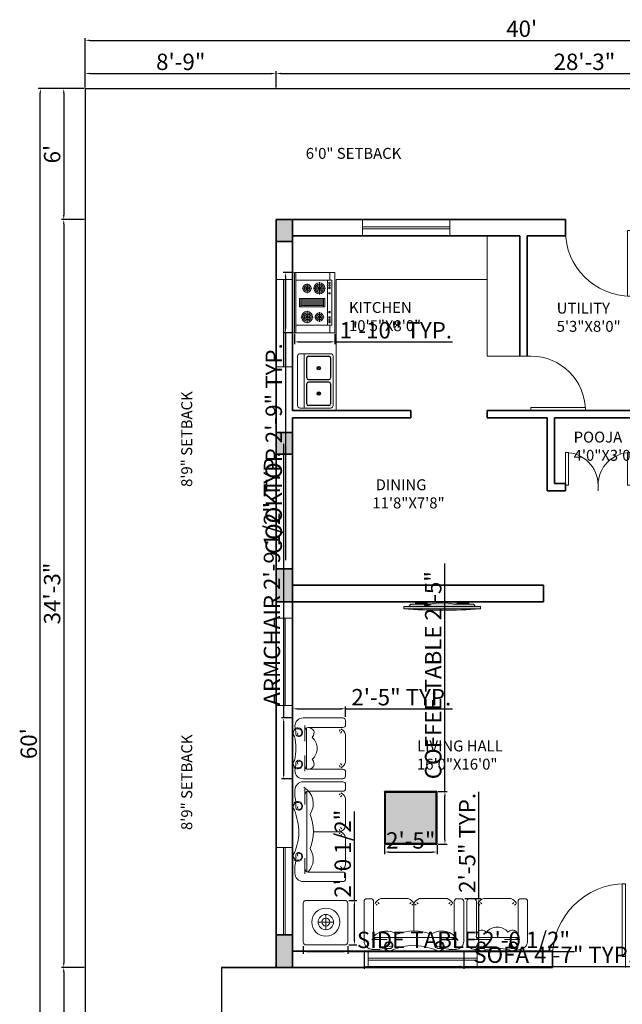
# Model space of a CAD drawing. Units: inches. Extents: x 3321 to 5237, y 11 to 1752.
# Tile 5 of 43: x 3321 to 3652, y 1204 to 1745. Entities that reach past the tile are written whole.
import ezdxf

# ---------------------------------------------------------------- set-up
doc = ezdxf.new("R2010")
doc.units = ezdxf.units.IN
for name, color, linetype, lineweight in [('A-ANNO-DIMS', 2, 'Continuous', 18), ('A-ANNO-TEXT', 7, 'Continuous', 18), ('A-AREA-IDEN', 7, 'Continuous', 18), ('A-COLS', 1, 'Continuous', 35), ('A-DOOR', 4, 'Continuous', 18), ('A-EQPM', 8, 'Continuous', 18), ('A-FLOR-CASE', 8, 'Continuous', 18), ('A-FLOR-EDGE', 7, 'Continuous', 25), ('A-GLAZ', 5, 'Continuous', 18), ('A-WALL', 7, 'Continuous', 35), ('C-PROP', 7, 'Continuous', 30), ('estofado', 7, 'Continuous', 25), ('FUR', 42, 'Continuous', 18), ('KITSHEN', 44, 'Continuous', 18), ('moveis', 254, 'Continuous', 5), ('parede', 7, 'Continuous', 30)]:
    doc.layers.add(name, color=color, linetype=linetype, lineweight=lineweight)
doc.layers.add('furn', color=17, linetype='Continuous')
doc.styles.get("Standard").update_dxf_attribs({"font": 'arial.ttf'})
doc.dimstyles.new('ISO-25', dxfattribs={"dimtxt": 9, "dimasz": 2.5, "dimexe": 1.25, "dimexo": 0.625, "dimtad": 1, "dimdec": 1, "dimlunit": 3, "dimtxsty": 'Standard', "dimcen": 2.5, "dimclrd": 4, "dimclre": 4, "dimclrt": 256, "dimadec": 0, "dimazin": 0, "dimtfac": 1, "dimtdec": 1, "dimtmove": 0, "dimatfit": 3, "dimfxl": 1, "dimarcsym": 0})

# ---------------------------------------------------------------- blocks, each defined once
blk = doc.blocks.new('*U2')
for p, q in [((0, 0), (0, -6)), ((-40, 0), (-40, -6))]:
    blk.add_line(p, q)
blk.add_lwpolyline([(0, 0), (0, 40), (-1.75, 40), (-1.75, 0)], close=True)
blk.add_arc((0, 0), 40, 90, 180)
blk = doc.blocks.new('*U5')
for p, q in [((0, 0), (0, -6)), ((-30, 0), (-30, -6))]:
    blk.add_line(p, q)
blk.add_lwpolyline([(0, 0), (0, 30), (-1.75, 30), (-1.75, 0)], close=True)
blk.add_arc((0, 0), 30, 90, 180)
blk = doc.blocks.new('*U11')
for p, q in [((0, 0), (0, -6)), ((36, 0), (36, -6))]:
    blk.add_line(p, q)
blk.add_lwpolyline([(0, 0), (0, 36), (1.75, 36), (1.75, 0)], close=True)
blk.add_arc((0, 0), 36, 0, 90)
blk = doc.blocks.new('*D30')
at = {"layer": 'A-ANNO-DIMS', "color": 0, "lineweight": -2, "transparency": 16777216}
for p, q in [((3356.06, 1707.34), (3343.59, 1707.34)), ((3344.84, 1704.84), (3344.84, 1637.84)), ((3356.06, 1635.34), (3343.59, 1635.34))]:
    blk.add_line(p, q, dxfattribs=at)
at = {"layer": 'A-ANNO-DIMS', "color": 0, "transparency": 16777216}
for points in [[(3344.42, 1704.84), (3345.26, 1704.84), (3344.84, 1707.34)], [(3344.42, 1637.84), (3345.26, 1637.84), (3344.84, 1635.34)]]:
    blk.add_solid(points, dxfattribs=at)
at = {"layer": 'Defpoints', "color": 0, "transparency": 16777216}
for p in [(3356.69, 1707.34), (3344.84, 1635.34), (3356.69, 1635.34)]:
    blk.add_point(p, dxfattribs=at)
at = {"layer": 'A-ANNO-DIMS', "color": 0, "transparency": 16777216, "insert": (3339.62, 1671.34), "char_height": 9, "attachment_point": 5, "rotation": 90}
blk.add_mtext("6'", dxfattribs=at)
blk = doc.blocks.new('*D31')
at = {"layer": 'A-ANNO-DIMS', "color": 0, "lineweight": -2, "transparency": 16777216}
for p, q in [((3356.06, 1635.34), (3343.59, 1635.34)), ((3344.84, 1632.84), (3344.84, 1226.84)), ((3356.06, 1224.34), (3343.59, 1224.34))]:
    blk.add_line(p, q, dxfattribs=at)
at = {"layer": 'A-ANNO-DIMS', "color": 0, "transparency": 16777216}
for points in [[(3344.42, 1632.84), (3345.26, 1632.84), (3344.84, 1635.34)], [(3344.42, 1226.84), (3345.26, 1226.84), (3344.84, 1224.34)]]:
    blk.add_solid(points, dxfattribs=at)
at = {"layer": 'Defpoints', "color": 0, "transparency": 16777216}
for p in [(3356.69, 1635.34), (3344.84, 1224.34), (3356.69, 1224.34)]:
    blk.add_point(p, dxfattribs=at)
at = {"layer": 'A-ANNO-DIMS', "color": 0, "transparency": 16777216, "insert": (3339.62, 1429.84), "char_height": 9, "attachment_point": 5, "rotation": 90}
blk.add_mtext('34\'-3"', dxfattribs=at)
blk = doc.blocks.new('*D32')
at = {"layer": 'A-ANNO-DIMS', "color": 0, "lineweight": -2, "transparency": 16777216}
for p, q in [((3356.06, 1224.34), (3343.59, 1224.34)), ((3344.84, 1221.84), (3344.84, 1034.84)), ((3356.06, 1032.34), (3343.59, 1032.34))]:
    blk.add_line(p, q, dxfattribs=at)
at = {"layer": 'A-ANNO-DIMS', "color": 0, "transparency": 16777216}
for points in [[(3344.42, 1221.84), (3345.26, 1221.84), (3344.84, 1224.34)], [(3344.42, 1034.84), (3345.26, 1034.84), (3344.84, 1032.34)]]:
    blk.add_solid(points, dxfattribs=at)
at = {"layer": 'Defpoints', "color": 0, "transparency": 16777216}
for p in [(3356.69, 1224.34), (3344.84, 1032.34), (3356.69, 1032.34)]:
    blk.add_point(p, dxfattribs=at)
at = {"layer": 'A-ANNO-DIMS', "color": 0, "transparency": 16777216, "insert": (3339.62, 1128.34), "char_height": 9, "attachment_point": 5, "rotation": 90}
blk.add_mtext("16'", dxfattribs=at)
blk = doc.blocks.new('*D38')
at = {"layer": 'A-ANNO-DIMS', "color": 0, "lineweight": -2, "transparency": 16777216}
for p, q in [((3356.69, 1707.96), (3356.69, 1716.91)), ((3359.19, 1715.66), (3459.19, 1715.66)), ((3461.69, 1707.96), (3461.69, 1716.91))]:
    blk.add_line(p, q, dxfattribs=at)
at = {"layer": 'A-ANNO-DIMS', "color": 0, "transparency": 16777216}
for points in [[(3359.19, 1716.08), (3359.19, 1715.25), (3356.69, 1715.66)], [(3459.19, 1716.08), (3459.19, 1715.25), (3461.69, 1715.66)]]:
    blk.add_solid(points, dxfattribs=at)
at = {"layer": 'Defpoints', "color": 0, "transparency": 16777216}
for p in [(3461.69, 1715.66), (3356.69, 1707.34), (3461.69, 1707.34)]:
    blk.add_point(p, dxfattribs=at)
at = {"layer": 'A-ANNO-DIMS', "color": 0, "transparency": 16777216, "insert": (3409.19, 1720.88), "char_height": 9, "attachment_point": 5}
blk.add_mtext('8\'-9"', dxfattribs=at)
blk = doc.blocks.new('*D39')
at = {"layer": 'A-ANNO-DIMS', "color": 0, "lineweight": -2, "transparency": 16777216}
for p, q in [((3461.69, 1707.96), (3461.69, 1716.91)), ((3464.19, 1715.66), (3798.19, 1715.66)), ((3800.69, 1707.96), (3800.69, 1716.91))]:
    blk.add_line(p, q, dxfattribs=at)
at = {"layer": 'A-ANNO-DIMS', "color": 0, "transparency": 16777216}
for points in [[(3464.19, 1716.08), (3464.19, 1715.25), (3461.69, 1715.66)], [(3798.19, 1716.08), (3798.19, 1715.25), (3800.69, 1715.66)]]:
    blk.add_solid(points, dxfattribs=at)
at = {"layer": 'Defpoints', "color": 0, "transparency": 16777216}
for p in [(3800.69, 1715.66), (3461.69, 1707.34), (3800.69, 1707.34)]:
    blk.add_point(p, dxfattribs=at)
at = {"layer": 'A-ANNO-DIMS', "color": 0, "transparency": 16777216, "insert": (3631.19, 1720.89), "char_height": 9, "attachment_point": 5}
blk.add_mtext('28\'-3"', dxfattribs=at)
blk = doc.blocks.new('*D44')
at = {"layer": 'A-ANNO-DIMS', "color": 0, "lineweight": -2, "transparency": 16777216}
for p, q in [((3356.69, 1707.96), (3356.69, 1735.11)), ((3359.19, 1733.86), (3834.19, 1733.86)), ((3836.69, 1707.96), (3836.69, 1735.11))]:
    blk.add_line(p, q, dxfattribs=at)
at = {"layer": 'A-ANNO-DIMS', "color": 0, "transparency": 16777216}
for points in [[(3359.19, 1734.28), (3359.19, 1733.45), (3356.69, 1733.86)], [(3834.19, 1734.28), (3834.19, 1733.45), (3836.69, 1733.86)]]:
    blk.add_solid(points, dxfattribs=at)
at = {"layer": 'Defpoints', "color": 0, "transparency": 16777216}
for p in [(3836.69, 1733.86), (3356.69, 1707.34), (3836.69, 1707.34)]:
    blk.add_point(p, dxfattribs=at)
at = {"layer": 'A-ANNO-DIMS', "color": 0, "transparency": 16777216, "insert": (3596.69, 1739.08), "char_height": 9, "attachment_point": 5}
blk.add_mtext("40'", dxfattribs=at)
blk = doc.blocks.new('*D45')
at = {"layer": 'A-ANNO-DIMS', "color": 0, "lineweight": -2, "transparency": 16777216}
for p, q in [((3356.06, 1707.34), (3330.71, 1707.34)), ((3331.96, 989.84), (3331.96, 1704.84)), ((3356.06, 987.34), (3330.71, 987.34))]:
    blk.add_line(p, q, dxfattribs=at)
at = {"layer": 'A-ANNO-DIMS', "color": 0, "transparency": 16777216}
for points in [[(3331.55, 1704.84), (3332.38, 1704.84), (3331.96, 1707.34)], [(3331.55, 989.84), (3332.38, 989.84), (3331.96, 987.34)]]:
    blk.add_solid(points, dxfattribs=at)
at = {"layer": 'Defpoints', "color": 0, "transparency": 16777216}
for p in [(3331.96, 1707.34), (3356.69, 1707.34), (3356.69, 987.34)]:
    blk.add_point(p, dxfattribs=at)
at = {"layer": 'A-ANNO-DIMS', "color": 0, "transparency": 16777216, "insert": (3326.74, 1347.34), "char_height": 9, "attachment_point": 5, "rotation": 90}
blk.add_mtext("60'", dxfattribs=at)
blk = doc.blocks.new('Oven Pln 001')
at = {"layer": 'KITSHEN'}
for p, q in [((2216.8, 1000.7), (2306.8, 1000.7)), ((2216.8, 942.7), (2216.8, 1000.7)), ((2306.8, 942.7), (2306.8, 1000.7)), ((2228.1, 993.2), (2216.8, 993.2)), ((2228.1, 996.2), (2295.5, 996.2)), ((2228.1, 942.7), (2228.1, 996.2)), ((2228.1, 990.1), (2295.5, 990.1)), ((2240.4, 968.6), (2240.4, 987)), ((2255.6, 984), (2267.9, 984)), ((2257.7, 950.3), (2257.7, 984)), ((2259.7, 984), (2259.7, 950.3)), ((2261.8, 950.3), (2261.8, 984)), ((2263.8, 984), (2263.8, 950.3)), ((2265.9, 950.3), (2265.9, 984)), ((2283.2, 970.6), (2283.2, 985)), ((2295.5, 996.2), (2295.5, 942.7)), ((2295.5, 993.2), (2306.8, 993.2)), ((2231.2, 977.8), (2249.6, 977.8)), ((2276, 977.8), (2290.4, 977.8)), ((2233.2, 959.4), (2247.6, 959.4)), ((2240.4, 952.2), (2240.4, 966.6)), ((2274, 959.4), (2292.4, 959.4)), ((2283.2, 950.2), (2283.2, 968.6)), ((2216.8, 940.7), (2216.8, 942.7)), ((2306.8, 942.7), (2216.8, 942.7)), ((2306.8, 940.7), (2216.8, 940.7)), ((2267.9, 950.3), (2255.6, 950.3)), ((2306.8, 940.7), (2306.8, 942.7))]:
    blk.add_line(p, q, dxfattribs=at)
blk.add_lwpolyline([(2255.6, 948.3), (2255.6, 986), (2267.9, 986), (2267.9, 948.3)], close=True, dxfattribs=at)
for centre, radius in [((2232.6, 992.9), 1.16), ((2240.4, 977.8), 8.19), ((2240.4, 977.8), 6.14), ((2236.1, 992.9), 1.16), ((2239.7, 992.9), 1.16), ((2247.7, 992.9), 1.16), ((2275.9, 992.9), 1.16), ((2283.2, 977.8), 6.14), ((2283.9, 992.9), 1.16), ((2287.5, 992.9), 1.16), ((2290.9, 992.9), 1.16), ((2240.4, 977.8), 4.09), ((2240.4, 977.8), 2.05), ((2283.2, 977.8), 4.09), ((2283.2, 977.8), 2.05), ((2240.4, 959.4), 6.14), ((2240.4, 959.4), 4.09), ((2240.4, 959.4), 2.05), ((2283.2, 959.4), 8.19), ((2283.2, 959.4), 6.14), ((2283.2, 959.4), 4.09), ((2283.2, 959.4), 2.05)]:
    blk.add_circle(centre, radius, dxfattribs=at)
blk = doc.blocks.new('ps sin 19')
at = {"layer": 'furn'}
for p, q in [((5312.3, 277.7), (5312.3, 306.3)), ((5314.6, 308.7), (5342.6, 308.7)), ((5345, 277.7), (5345, 306.3)), ((5348.6, 306.3), (5348.6, 277.7)), ((5350.9, 308.7), (5378.9, 308.7)), ((5381.3, 306.3), (5381.3, 277.7)), ((5342.6, 275.3), (5314.6, 275.3)), ((5378.9, 275.3), (5350.9, 275.3))]:
    blk.add_line(p, q, dxfattribs=at)
for centre, radius in [((5328.9, 292), 2.38), ((5328.9, 292), 1.19), ((5364.6, 292), 2.38), ((5364.6, 292), 1.19)]:
    blk.add_circle(centre, radius, dxfattribs=at)
for centre, start, end in [((5314.6, 306.3), 90, 180), ((5342.6, 306.3), 0, 90), ((5350.9, 306.3), 90, 180), ((5378.9, 306.3), 0, 90), ((5314.6, 277.7), 180, 270), ((5342.6, 277.7), 270, 0), ((5350.9, 277.7), 180, 270), ((5378.9, 277.7), 270, 0)]:
    blk.add_arc(centre, 2.38, start, end, dxfattribs=at)
at = {"layer": 'KITSHEN'}
for p, q in [((5308.7, 275.3), (5308.7, 318.2)), ((5312.3, 321.8), (5381.3, 321.8)), ((5384.9, 318.2), (5384.9, 275.3)), ((5308.7, 312.2), (5384.9, 312.2)), ((5381.3, 271.8), (5312.3, 271.8))]:
    blk.add_line(p, q, dxfattribs=at)
for centre, start, end in [((5312.3, 318.2), 90, 180), ((5381.3, 318.2), 0, 90), ((5312.3, 275.3), 180, 270), ((5381.3, 275.3), 270, 0)]:
    blk.add_arc(centre, 3.57, start, end, dxfattribs=at)
blk = doc.blocks.new('sofa-34')
at = {"color": 0, "linetype": 'ByBlock'}
for p, q in [((-0.026, 0.924), (-0.1, 0.924)), ((0.657, 0.925), (0.153, 0.925)), ((0.836, 0.924), (0.91, 0.924)), ((-0.15, 0.15), (-0.15, 0.874)), ((0.024, 0.236), (0.024, 0.874)), ((0.05, 0.838), (0.05, 0.838)), ((0.09, 0.806), (0.068, 0.824)), ((0.101, 0.857), (0.126, 0.829)), ((0.71, 0.857), (0.684, 0.829)), ((0.72, 0.806), (0.742, 0.824)), ((0.76, 0.838), (0.76, 0.838)), ((0.76, 0.838), (0.76, 0.838)), ((0.786, 0.236), (0.786, 0.874)), ((0.96, 0.15), (0.96, 0.874)), ((-0.01, 0.18), (0.274, 0.18)), ((0.029, 0.214), (0.781, 0.214)), ((0.82, 0.18), (0.536, 0.18))]:
    blk.add_line(p, q, dxfattribs=at)
blk.add_arc((0.405, 0.148), 0.258, 40.7983, 139.2017, dxfattribs=at)
at = {"color": 0, "linetype": 'ByBlock', "extrusion": (0, 0, -1)}
for centre, major_axis, ratio, start_param, end_param in [((-0.1, 0.874), (0.0354, 0.0354), 1, 3.926992, 5.497787), ((-0.026, 0.874), (-0.0354, 0.0354), 1, 0.785398, 2.356196), ((0.2, 0.766), (0.117, 0.117), 1, 4.372209, 5.213218), ((0.61, 0.766), (0.117, 0.117), 1, -0.500829, 0.34018), ((0.5, -0.587), (-0.415, 0.931), 0.264583, -0.381915, 0.387685), ((0.074, 0.236), (-0.0354, 0.0354), 1, 3.926991, 5.497788), ((0, 0.15), (0.106, 0.106), 1, 2.356194, 3.926992), ((0.179, -0.658), (-0.251, 0.635), 0.885019, 0.124301, 0.339591), ((0.117, 0.052), (-0.0624, 0.0624), 1, 4.675944, 7.152385), ((0.13, 0.052), (-0.059, 0.059), 1, 3.186406, 6.094039), ((0.114, 0.063), (-0.0458, 0.0458), 1, 6.094039, 8.043134), ((0.129, 0.073), (-0.0414, 0.0414), 1, 2.230507, 4.423483), ((0.139, 0.08), (0.0245, 0.0245), 1, 0.189152, 2.952444), ((0.118, 0.071), (0.0491, 0.0491), 1, -0.701597, 0.659711), ((0.352, -0.558), (0.735, 0.107), 0.76838, 4.597815, 5.20076)]:
    blk.add_ellipse(centre, major_axis=major_axis, ratio=ratio, start_param=start_param, end_param=end_param, dxfattribs=at)
at = {"color": 0, "linetype": 'ByBlock'}
for centre, major_axis, ratio, start_param, end_param in [((0.836, 0.874), (0.0354, 0.0354), 1, 0.785398, 2.356196), ((0.91, 0.874), (-0.0354, 0.0354), 1, 3.926992, 5.497787), ((0.31, -0.587), (0.415, 0.931), 0.264583, -0.381915, 0.387685), ((0.736, 0.236), (0.0354, 0.0354), 1, 3.926991, 5.497788), ((0.681, 0.073), (0.0414, 0.0414), 1, 2.230507, 4.423483), ((0.692, 0.071), (-0.0491, 0.0491), 1, -0.701597, 0.659711), ((0.68, 0.052), (0.059, 0.059), 1, 3.186406, 6.094039), ((0.671, 0.08), (-0.0245, 0.0245), 1, 0.189152, 2.952444), ((0.696, 0.063), (0.0458, 0.0458), 1, 6.094039, 8.043134), ((0.631, -0.658), (0.251, 0.635), 0.885019, 0.124301, 0.339591), ((0.693, 0.052), (0.0624, 0.0624), 1, 4.675944, 7.152385), ((0.81, 0.15), (-0.106, 0.106), 1, 2.356194, 3.926992)]:
    blk.add_ellipse(centre, major_axis=major_axis, ratio=ratio, start_param=start_param, end_param=end_param, dxfattribs=at)
blk = doc.blocks.new('sofa-33')
at = {"color": 0, "linetype": 'ByBlock'}
for p, q in [((-0.026, 0.924), (-0.1, 0.924)), ((0.657, 0.925), (0.153, 0.925)), ((0.863, 0.925), (1.367, 0.925)), ((1.62, 0.924), (1.546, 0.924)), ((-0.15, 0.15), (-0.15, 0.874)), ((0.024, 0.236), (0.024, 0.874)), ((0.05, 0.838), (0.05, 0.838)), ((0.09, 0.806), (0.068, 0.824)), ((0.101, 0.857), (0.126, 0.829)), ((0.71, 0.857), (0.684, 0.829)), ((0.72, 0.806), (0.742, 0.824)), ((0.76, 0.838), (0.76, 0.336)), ((0.76, 0.838), (0.76, 0.838)), ((0.76, 0.838), (0.76, 0.838)), ((0.8, 0.806), (0.778, 0.824)), ((0.811, 0.857), (0.837, 0.829)), ((1.42, 0.857), (1.394, 0.829)), ((1.43, 0.806), (1.452, 0.824)), ((1.47, 0.838), (1.47, 0.838)), ((1.47, 0.838), (1.47, 0.838)), ((1.496, 0.236), (1.496, 0.874)), ((1.67, 0.15), (1.67, 0.874)), ((-0.01, 0.18), (0.274, 0.18)), ((0.029, 0.214), (1.491, 0.214)), ((1.542, 0.18), (1.258, 0.18)), ((0, 0), (0.136, 0)), ((1.532, 0), (1.397, 0))]:
    blk.add_line(p, q, dxfattribs=at)
at = {"color": 0, "linetype": 'ByBlock', "extrusion": (0, 0, -1)}
for centre, major_axis, ratio, start_param, end_param in [((-0.1, 0.874), (0.0354, 0.0354), 1, 3.926992, 5.497787), ((-0.026, 0.874), (-0.0354, 0.0354), 1, 0.785398, 2.356196), ((0.2, 0.766), (0.117, 0.117), 1, 4.372209, 5.213218), ((0.61, 0.766), (0.117, 0.117), 1, -0.500829, 0.34018), ((0.91, 0.766), (0.117, 0.117), 1, 4.372209, 5.213218), ((1.321, 0.766), (-0.117, 0.117), 1, 1.069968, 1.910976), ((1.546, 0.874), (-0.0354, 0.0354), 1, 5.497786, 7.068583), ((1.62, 0.874), (0.0354, 0.0354), 1, -0.785398, 0.785398), ((0.323, -0.666), (-0.093, 1), 0.551284, -0.397889, 0.397889), ((1.147, -0.534), (0.2, 0.861), 0.59532, -0.502747, 0.502747), ((0.074, 0.236), (-0.0354, 0.0354), 1, 3.926991, 5.497788), ((0.766, -0.668), (-0.003, 1.004), 0.922365, -0.343589, 0.343589), ((1.446, 0.236), (0.0354, 0.0354), 1, 0.785397, 2.356194), ((0, 0.15), (0.106, 0.106), 1, 2.356194, 3.926992), ((0.282, -0.661), (-0.479, 0.479), 1, 0.566947, 0.842011), ((0.308, 0.052), (-0.0624, 0.0624), 1, 4.675944, 7.152385), ((0.321, 0.052), (-0.059, 0.059), 1, 3.186406, 6.094039), ((0.305, 0.063), (-0.0458, 0.0458), 1, 6.094039, 8.043134), ((0.32, 0.073), (-0.0414, 0.0414), 1, 2.230507, 4.423483), ((0.33, 0.08), (0.0245, 0.0245), 1, 0.189152, 2.952444), ((0.309, 0.071), (0.0491, 0.0491), 1, -0.701597, 0.659711), ((0.878, -1.382), (-0.323, 1.429), 0.878591, -0.144977, 0.144977), ((0.667, -1.39), (1.036, 1.036), 1, 5.547613, 5.837566), ((1.212, 0.073), (-0.0414, 0.0414), 1, 3.430501, 5.623477), ((1.223, 0.071), (-0.0491, 0.0491), 1, 5.623477, 6.984784), ((1.211, 0.052), (0.059, 0.059), 1, 0.189149, 3.096782), ((1.202, 0.08), (0.0245, 0.0245), 1, 1.759947, 4.52324), ((1.227, 0.063), (0.0458, 0.0458), 1, 4.52324, 6.472335), ((1.25, -0.661), (0.479, 0.479), 1, 5.441177, 5.716241), ((1.225, 0.052), (-0.0624, 0.0624), 1, 0.701599, 3.17804), ((1.52, 0.15), (0.106, 0.106), 1, 0.785398, 2.356194)]:
    blk.add_ellipse(centre, major_axis=major_axis, ratio=ratio, start_param=start_param, end_param=end_param, dxfattribs=at)
blk = doc.blocks.new('table-31')
at = {"color": 0, "linetype": 'ByBlock'}
for p, q in [((0.1683, 0.1952), (-0.1746, 0.1952)), ((-0.2031, 0.1666), (-0.2031, -0.1763)), ((0.1969, 0.1666), (0.1969, -0.1763)), ((-0.0689, 0), (0.0689, 0)), ((0, -0.0689), (0, 0.0689)), ((0.1683, -0.2048), (-0.1746, -0.2048))]:
    blk.add_line(p, q, dxfattribs=at)
for radius in [0.1261, 0.0689, 0.0353]:
    blk.add_circle((0, 0), radius, dxfattribs=at)
for centre, start, end in [((-0.1746, 0.1666), 90, 180), ((0.1683, 0.1666), 0, 90), ((-0.1746, -0.1763), 180, 270), ((0.1683, -0.1763), 270, 0)]:
    blk.add_arc(centre, 0.0286, start, end, dxfattribs=at)
blk = doc.blocks.new('Mesa Espelho reflex microtubos')
at = {"layer": 'estofado', "ltscale": 0.5}
h = blk.add_hatch(color=256, dxfattribs=at)
h.dxf.hatch_style = 1
h.set_gradient(color1=(219, 219, 220), one_color=1, tint=1, name='CYLINDER')
h.paths.add_polyline_path([(0.605, 0), (-0.605, 0), (-0.585, -0.02), (0.585, -0.02)])
h.paths.add_polyline_path([(-0.585, -0.02), (-0.605, 0), (-0.605, -1.21), (-0.585, -1.19)])
h.paths.add_polyline_path([(0.605, 0), (0.585, -0.02), (0.585, -1.19), (0.605, -1.21)])
h.paths.add_polyline_path([(0.585, -1.19), (-0.585, -1.19), (-0.605, -1.21), (0.605, -1.21)])
h = blk.add_hatch(color=256, dxfattribs=at)
h.dxf.hatch_style = 1
h.set_gradient(color1=(219, 219, 220), one_color=1, tint=1, name='CYLINDER')
h.paths.add_polyline_path([(0.585, -0.02), (-0.585, -0.02), (-0.585, -1.19), (0.585, -1.19)])
for p, q in [((-0.585, -0.02), (-0.605, 0)), ((0.585, -0.02), (0.605, 0)), ((-0.585, -1.19), (-0.605, -1.21)), ((0.585, -1.19), (0.605, -1.21))]:
    blk.add_line(p, q, dxfattribs=at)
for points in [[(-0.605, -1.21), (0.605, -1.21), (0.605, 0), (-0.605, 0)], [(-0.585, -1.19), (0.585, -1.19), (0.585, -0.02), (-0.585, -0.02)]]:
    blk.add_lwpolyline(points, close=True, dxfattribs=at)
blk = doc.blocks.new('PLASMA 2')
at = {"layer": 'moveis', "ltscale": 0.08}
h = blk.add_hatch(dxfattribs=at)
h.set_pattern_fill('_USER,_O', color=256, scale=0.008, double=1, pattern_type=0)
h.set_pattern_definition([(360, (-4.134502, -6.848382), (0, 0.008), []), (90, (-4.134502, -6.848382), (-0.008, 0), [])])
h.paths.add_polyline_path([(-0.21, -0.097), (-0.362, -0.097), (-0.362, -0.111), (-0.21, -0.111)])
h = blk.add_hatch(dxfattribs=at)
h.set_pattern_fill('_USER,_O', color=256, scale=0.008, double=1, pattern_type=0)
h.set_pattern_definition([(180, (4.134502, -6.848382), (0, 0.008), []), (90, (4.134502, -6.848382), (0.008, 0), [])])
h.paths.add_polyline_path([(0.21, -0.097), (0.362, -0.097), (0.362, -0.111), (0.21, -0.111)])
at = {"layer": 'parede', "ltscale": 0.08}
h = blk.add_hatch(color=256, dxfattribs=at)
h.dxf.hatch_style = 1
h.set_gradient(color1=(131, 136, 145), one_color=1, tint=1, name='CURVED')
h.paths.add_polyline_path([(-0.535, -0.022), (0.535, -0.022, 0.040195)])
h = blk.add_hatch(color=256, dxfattribs=at)
h.dxf.hatch_style = 1
h.set_gradient(color1=(131, 136, 145), color2=(0, 0, 0), one_color=1, name='CURVED')
h.paths.add_polyline_path([(0.535, -0.022), (-0.535, -0.022), (-0.535, -0.055), (0.535, -0.055)])
h = blk.add_hatch(color=256, dxfattribs=at)
h.dxf.hatch_style = 1
h.set_gradient(color1=(131, 136, 145), one_color=1, tint=1, name='CYLINDER')
h.paths.add_polyline_path([(0.467, -0.055), (-0.467, -0.055), (-0.436, -0.088), (-0.164, -0.088, 0.114423), (0.164, -0.088), (0.436, -0.088)])
h = blk.add_hatch(color=256, dxfattribs=at)
h.dxf.hatch_style = 1
h.set_gradient(color1=(131, 136, 145), color2=(0, 0, 0), one_color=1, name='CURVED')
h.paths.add_polyline_path([(0.372, -0.088), (0.164, -0.088, -0.114423), (-0.164, -0.088), (-0.372, -0.088), (-0.372, -0.12), (0.372, -0.12)])
h.paths.add_polyline_path([(-0.21, -0.111), (-0.362, -0.111), (-0.362, -0.097), (-0.21, -0.097)], flags=16)
h.paths.add_polyline_path([(0.21, -0.111), (0.21, -0.097), (0.362, -0.097), (0.362, -0.111)], flags=16)
at = {"layer": 'moveis', "ltscale": 0.08}
for p, q in [((-0.535, -0.022), (-0.535, -0.055)), ((-0.535, -0.022), (0.535, -0.022)), ((0.535, -0.055), (-0.535, -0.055)), ((-0.467, -0.055), (-0.436, -0.088)), ((-0.436, -0.088), (-0.164, -0.088)), ((-0.372, -0.088), (-0.372, -0.12)), ((-0.372, -0.12), (0.372, -0.12)), ((0.164, -0.088), (0.436, -0.088)), ((0.372, -0.088), (0.372, -0.12)), ((0.467, -0.055), (0.436, -0.088)), ((0.535, -0.055), (0.535, -0.022))]:
    blk.add_line(p, q, dxfattribs=at)
for points in [[(-0.362, -0.097), (-0.21, -0.097), (-0.21, -0.111), (-0.362, -0.111)], [(0.362, -0.097), (0.21, -0.097), (0.21, -0.111), (0.362, -0.111)]]:
    blk.add_lwpolyline(points, close=True, dxfattribs=at)
for centre, radius, start, end in [((0, -6.666), 6.666, 85.3965, 94.6035), ((0, 0.618), 0.724, 256.9449, 283.0551)]:
    blk.add_arc(centre, radius, start, end, dxfattribs=at)
blk = doc.blocks.new('COL-9X18-IN')
h = blk.add_hatch(color=256)
h.dxf.hatch_style = 1
h.paths.add_polyline_path([(9, 18), (0, 18), (0, 0), (9, 0)])
blk.add_lwpolyline([(0, 0), (9, 0), (9, 18), (0, 18)], close=True)
blk = doc.blocks.new('COL-9X12-FURN-PLAN')
h = blk.add_hatch(color=256)
h.dxf.hatch_style = 1
h.paths.add_polyline_path([(0, 12), (0, 0), (9, 0), (9, 12)])
blk.add_lwpolyline([(0, 0), (9, 0), (9, 12), (0, 12)], close=True)
blk = doc.blocks.new('WIN-48IN-9IN-WALL')
for p, q in [((0, 0), (0, 9)), ((48, 0), (48, 9)), ((0, 5), (48, 5)), ((0, 4), (48, 4))]:
    blk.add_line(p, q)
blk = doc.blocks.new('WIN-60IN-9IN-WALL')
for p, q in [((0, 0), (0, 9)), ((60, 0), (60, 9)), ((0, 5), (60, 5)), ((0, 4), (60, 4))]:
    blk.add_line(p, q)
blk = doc.blocks.new('DOOR-DOUBLE-36IN')
for p, q in [((0, 3), (0, 0)), ((18, 3), (18, 0)), ((18, 3), (18, 0)), ((36, 3), (36, 0))]:
    blk.add_line(p, q)
for points in [[(0, 3), (0, 21), (1.75, 21), (1.75, 3)], [(36, 3), (36, 21), (34.25, 21), (34.25, 3)]]:
    blk.add_lwpolyline(points, close=True)
for centre, start, end in [((0, 3), 0, 90), ((36, 3), 90, 180)]:
    blk.add_arc(centre, 18, start, end)
blk = doc.blocks.new('PROPERTY-40X60FT')
for q in [(480, 720), (0, 0)]:
    blk.add_line((0, 720), q)
blk = doc.blocks.new('*D203')
at = {"layer": 'A-ANNO-DIMS', "color": 4, "lineweight": -2, "transparency": 16777216}
for p, q in [((3465.79, 1361.47), (3465.79, 1512.12)), ((3470.19, 1361.47), (3464.54, 1361.47)), ((3465.79, 1330.51), (3465.79, 1358.97)), ((3470.19, 1328.01), (3464.54, 1328.01))]:
    blk.add_line(p, q, dxfattribs=at)
at = {"layer": 'A-ANNO-DIMS', "color": 4, "transparency": 16777216}
for points in [[(3465.38, 1358.97), (3466.21, 1358.97), (3465.79, 1361.47)], [(3465.38, 1330.51), (3466.21, 1330.51), (3465.79, 1328.01)]]:
    blk.add_solid(points, dxfattribs=at)
at = {"layer": 'Defpoints', "color": 0, "transparency": 16777216}
for p in [(3465.79, 1361.47), (3470.81, 1361.47), (3470.81, 1328.01)]:
    blk.add_point(p, dxfattribs=at)
at = {"layer": 'A-ANNO-DIMS', "transparency": 16777216, "insert": (3460.51, 1438.04), "char_height": 9, "attachment_point": 5, "rotation": 90}
blk.add_mtext('ARMCHAIR 2\'-9 1/2" TYP.', dxfattribs=at)
blk = doc.blocks.new('*D204')
at = {"layer": 'A-ANNO-DIMS', "color": 4, "lineweight": -2, "transparency": 16777216}
for p, q in [((3470.81, 1362.09), (3470.81, 1367.73)), ((3473.31, 1366.48), (3497.35, 1366.48)), ((3499.85, 1362.09), (3499.85, 1367.73)), ((3499.85, 1366.48), (3558.61, 1366.48))]:
    blk.add_line(p, q, dxfattribs=at)
at = {"layer": 'A-ANNO-DIMS', "color": 4, "transparency": 16777216}
for points in [[(3473.31, 1366.9), (3473.31, 1366.07), (3470.81, 1366.48)], [(3497.35, 1366.9), (3497.35, 1366.07), (3499.85, 1366.48)]]:
    blk.add_solid(points, dxfattribs=at)
at = {"layer": 'Defpoints', "color": 0, "transparency": 16777216}
for p in [(3499.85, 1366.48), (3470.81, 1361.47), (3499.85, 1361.47)]:
    blk.add_point(p, dxfattribs=at)
at = {"layer": 'A-ANNO-DIMS', "transparency": 16777216, "insert": (3530.48, 1371.7), "char_height": 9, "attachment_point": 5}
blk.add_mtext('2\'-5" TYP.', dxfattribs=at)
blk = doc.blocks.new('*D207')
at = {"layer": 'A-ANNO-DIMS', "color": 4, "lineweight": -2, "transparency": 16777216}
for p, q in [((3510, 1232.49), (3510, 1223.64)), ((3564.86, 1232.49), (3564.86, 1223.64)), ((3512.5, 1224.89), (3562.36, 1224.89)), ((3564.86, 1224.89), (3661.15, 1224.89))]:
    blk.add_line(p, q, dxfattribs=at)
at = {"layer": 'A-ANNO-DIMS', "color": 4, "transparency": 16777216}
for points in [[(3512.5, 1225.31), (3512.5, 1224.47), (3510, 1224.89)], [(3562.36, 1225.31), (3562.36, 1224.47), (3564.86, 1224.89)]]:
    blk.add_solid(points, dxfattribs=at)
at = {"layer": 'Defpoints', "color": 0, "transparency": 16777216}
for p in [(3510, 1233.12), (3564.86, 1233.12), (3564.86, 1224.89)]:
    blk.add_point(p, dxfattribs=at)
at = {"layer": 'A-ANNO-DIMS', "transparency": 16777216, "insert": (3614.25, 1230.17), "char_height": 9, "attachment_point": 5}
blk.add_mtext('SOFA 4\'-7" TYP.', dxfattribs=at)
blk = doc.blocks.new('*D208')
at = {"layer": 'A-ANNO-DIMS', "color": 4, "lineweight": -2, "transparency": 16777216}
for p, q in [((3573.08, 1262.16), (3573.08, 1320.92)), ((3565.48, 1262.16), (3574.33, 1262.16)), ((3573.08, 1235.62), (3573.08, 1259.66)), ((3565.48, 1233.12), (3574.33, 1233.12))]:
    blk.add_line(p, q, dxfattribs=at)
at = {"layer": 'A-ANNO-DIMS', "color": 4, "transparency": 16777216}
for points in [[(3572.67, 1259.66), (3573.5, 1259.66), (3573.08, 1262.16)], [(3572.67, 1235.62), (3573.5, 1235.62), (3573.08, 1233.12)]]:
    blk.add_solid(points, dxfattribs=at)
at = {"layer": 'Defpoints', "color": 0, "transparency": 16777216}
for p in [(3564.86, 1262.16), (3573.08, 1262.16), (3564.86, 1233.12)]:
    blk.add_point(p, dxfattribs=at)
at = {"layer": 'A-ANNO-DIMS', "transparency": 16777216, "insert": (3567.86, 1292.79), "char_height": 9, "attachment_point": 5, "rotation": 90}
blk.add_mtext('2\'-5" TYP.', dxfattribs=at)
blk = doc.blocks.new('*D211')
at = {"layer": 'A-ANNO-DIMS', "color": 4, "lineweight": -2, "transparency": 16777216}
for p, q in [((3476.53, 1236.07), (3476.53, 1231.77)), ((3501.04, 1236.07), (3501.04, 1231.77)), ((3479.03, 1233.02), (3498.54, 1233.02)), ((3501.04, 1233.02), (3625.8, 1233.02))]:
    blk.add_line(p, q, dxfattribs=at)
at = {"layer": 'A-ANNO-DIMS', "color": 4, "transparency": 16777216}
for points in [[(3479.03, 1233.44), (3479.03, 1232.6), (3476.53, 1233.02)], [(3498.54, 1233.44), (3498.54, 1232.6), (3501.04, 1233.02)]]:
    blk.add_solid(points, dxfattribs=at)
at = {"layer": 'Defpoints', "color": 0, "transparency": 16777216}
for p in [(3476.53, 1236.7), (3501.04, 1236.7), (3501.04, 1233.02)]:
    blk.add_point(p, dxfattribs=at)
at = {"layer": 'A-ANNO-DIMS', "transparency": 16777216, "insert": (3564.67, 1238.3), "char_height": 9, "attachment_point": 5}
blk.add_mtext('SIDE TABLE 2\'-0 1/2"', dxfattribs=at)
blk = doc.blocks.new('*D212')
at = {"layer": 'A-ANNO-DIMS', "color": 4, "lineweight": -2, "transparency": 16777216}
for p, q in [((3504.71, 1261.2), (3504.71, 1310)), ((3501.66, 1261.2), (3505.96, 1261.2)), ((3504.71, 1239.2), (3504.71, 1258.7)), ((3501.66, 1236.7), (3505.96, 1236.7))]:
    blk.add_line(p, q, dxfattribs=at)
at = {"layer": 'A-ANNO-DIMS', "color": 4, "transparency": 16777216}
for points in [[(3504.29, 1258.7), (3505.13, 1258.7), (3504.71, 1261.2)], [(3504.29, 1239.2), (3505.13, 1239.2), (3504.71, 1236.7)]]:
    blk.add_solid(points, dxfattribs=at)
at = {"layer": 'Defpoints', "color": 0, "transparency": 16777216}
for p in [(3501.04, 1261.2), (3504.71, 1261.2), (3501.04, 1236.7)]:
    blk.add_point(p, dxfattribs=at)
at = {"layer": 'A-ANNO-DIMS', "transparency": 16777216, "insert": (3499.43, 1286.85), "char_height": 9, "attachment_point": 5, "rotation": 90}
blk.add_mtext('2\'-0 1/2"', dxfattribs=at)
blk = doc.blocks.new('*D217')
at = {"layer": 'A-ANNO-DIMS', "color": 4, "lineweight": -2, "transparency": 16777216}
for p, q in [((3471.14, 1606.27), (3465.54, 1606.27)), ((3466.79, 1603.77), (3466.79, 1575.62)), ((3471.14, 1573.12), (3465.54, 1573.12)), ((3466.79, 1573.12), (3466.79, 1448.25))]:
    blk.add_line(p, q, dxfattribs=at)
at = {"layer": 'A-ANNO-DIMS', "color": 4, "transparency": 16777216}
for points in [[(3466.37, 1603.77), (3467.21, 1603.77), (3466.79, 1606.27)], [(3466.37, 1575.62), (3467.21, 1575.62), (3466.79, 1573.12)]]:
    blk.add_solid(points, dxfattribs=at)
at = {"layer": 'Defpoints', "color": 0, "transparency": 16777216}
for p in [(3471.76, 1606.27), (3466.79, 1573.12), (3471.76, 1573.12)]:
    blk.add_point(p, dxfattribs=at)
at = {"layer": 'A-ANNO-DIMS', "transparency": 16777216, "insert": (3461.51, 1509.43), "char_height": 9, "attachment_point": 5, "rotation": 90}
blk.add_mtext('COOKTOP 2\'-9" TYP.', dxfattribs=at)
blk = doc.blocks.new('*D218')
at = {"layer": 'A-ANNO-DIMS', "color": 4, "lineweight": -2, "transparency": 16777216}
for p, q in [((3471.76, 1572.49), (3471.76, 1566.9)), ((3493.88, 1572.49), (3493.88, 1566.9)), ((3474.26, 1568.15), (3491.38, 1568.15)), ((3493.88, 1568.15), (3558.63, 1568.15))]:
    blk.add_line(p, q, dxfattribs=at)
at = {"layer": 'A-ANNO-DIMS', "color": 4, "transparency": 16777216}
for points in [[(3474.26, 1568.56), (3474.26, 1567.73), (3471.76, 1568.15)], [(3491.38, 1568.56), (3491.38, 1567.73), (3493.88, 1568.15)]]:
    blk.add_solid(points, dxfattribs=at)
at = {"layer": 'Defpoints', "color": 0, "transparency": 16777216}
for p in [(3471.76, 1573.12), (3493.88, 1573.12), (3493.88, 1568.15)]:
    blk.add_point(p, dxfattribs=at)
at = {"layer": 'A-ANNO-DIMS', "transparency": 16777216, "insert": (3527.51, 1573.37), "char_height": 9, "attachment_point": 5}
blk.add_mtext('1\'-10" TYP.', dxfattribs=at)
blk = doc.blocks.new('*D221')
at = {"layer": 'A-ANNO-DIMS', "color": 4, "lineweight": -2, "transparency": 16777216}
for p, q in [((3554.47, 1321.02), (3554.47, 1446.4)), ((3550.75, 1321.02), (3555.72, 1321.02)), ((3554.47, 1294.6), (3554.47, 1318.52)), ((3550.75, 1292.1), (3555.72, 1292.1))]:
    blk.add_line(p, q, dxfattribs=at)
at = {"layer": 'A-ANNO-DIMS', "color": 4, "transparency": 16777216}
for points in [[(3554.05, 1318.52), (3554.88, 1318.52), (3554.47, 1321.02)], [(3554.05, 1294.6), (3554.88, 1294.6), (3554.47, 1292.1)]]:
    blk.add_solid(points, dxfattribs=at)
at = {"layer": 'Defpoints', "color": 0, "transparency": 16777216}
for p in [(3550.13, 1321.02), (3554.47, 1321.02), (3550.13, 1292.1)]:
    blk.add_point(p, dxfattribs=at)
at = {"layer": 'A-ANNO-DIMS', "transparency": 16777216, "insert": (3549.18, 1384.96), "char_height": 9, "attachment_point": 5, "rotation": 90}
blk.add_mtext('COFFEE TABLE 2\'-5"', dxfattribs=at)
blk = doc.blocks.new('*D222')
at = {"layer": 'A-ANNO-DIMS', "color": 4, "lineweight": -2, "transparency": 16777216}
for p, q in [((3521.21, 1291.47), (3521.21, 1286.51)), ((3550.13, 1291.47), (3550.13, 1286.51)), ((3523.71, 1287.76), (3547.63, 1287.76))]:
    blk.add_line(p, q, dxfattribs=at)
at = {"layer": 'A-ANNO-DIMS', "color": 4, "transparency": 16777216}
for points in [[(3523.71, 1288.17), (3523.71, 1287.34), (3521.21, 1287.76)], [(3547.63, 1288.17), (3547.63, 1287.34), (3550.13, 1287.76)]]:
    blk.add_solid(points, dxfattribs=at)
at = {"layer": 'Defpoints', "color": 0, "transparency": 16777216}
for p in [(3521.21, 1292.1), (3550.13, 1292.1), (3550.13, 1287.76)]:
    blk.add_point(p, dxfattribs=at)
at = {"layer": 'A-ANNO-DIMS', "transparency": 16777216, "insert": (3535.67, 1292.98), "char_height": 9, "attachment_point": 5}
blk.add_mtext('2\'-5"', dxfattribs=at)

msp = doc.modelspace()

# ---------------------------------------------------------------- linework, layer by layer
at = {"layer": 'A-FLOR-CASE'}
for p, q in [((3577.69, 1626.34), (3577.69, 1560.34)), ((3494.69, 1602.34), (3494.69, 1530.34)), ((3494.69, 1602.34), (3577.69, 1602.34)), ((3577.69, 1560.34), (3599.69, 1560.34))]:
    msp.add_line(p, q, dxfattribs=at)
at = {"layer": 'A-FLOR-EDGE'}
msp.add_line((3431.69, 1224.34), (3431.69, 1032.34), dxfattribs=at)
at = {"layer": 'A-WALL'}
for p, q in [((3461.69, 1635.34), (3461.69, 1224.34)), ((3461.69, 1635.34), (3620.69, 1635.34)), ((3620.69, 1635.34), (3620.69, 1626.34)), ((3470.69, 1626.34), (3595.69, 1626.34)), ((3470.69, 1626.34), (3470.69, 1530.34)), ((3595.69, 1626.34), (3595.69, 1560.34)), ((3599.69, 1626.34), (3599.69, 1560.34)), ((3599.69, 1626.34), (3620.69, 1626.34)), ((3470.69, 1530.34), (3535.69, 1530.34)), ((3470.69, 1526.34), (3535.69, 1526.34)), ((3470.69, 1526.34), (3470.69, 1434.34)), ((3535.69, 1530.34), (3535.69, 1526.34)), ((3577.69, 1530.34), (3577.69, 1526.34)), ((3577.69, 1530.34), (3662.69, 1530.34)), ((3577.69, 1526.34), (3610.69, 1526.34)), ((3610.69, 1526.34), (3610.69, 1486.34)), ((3614.69, 1526.34), (3614.69, 1490.34)), ((3614.69, 1526.34), (3662.69, 1526.34)), ((3614.69, 1490.34), (3620.69, 1490.34)), ((3620.69, 1490.34), (3620.69, 1486.34)), ((3610.69, 1486.34), (3620.69, 1486.34)), ((3470.69, 1434.34), (3608.69, 1434.34)), ((3608.69, 1434.34), (3608.69, 1425.34)), ((3470.69, 1425.34), (3608.69, 1425.34)), ((3470.69, 1425.34), (3470.69, 1233.34)), ((3470.69, 1233.34), (3613.69, 1233.34)), ((3613.69, 1233.34), (3613.69, 1224.34)), ((3431.69, 1224.34), (3613.69, 1224.34))]:
    msp.add_line(p, q, dxfattribs=at)

# ---------------------------------------------------------------- block references
at = {"layer": 'A-COLS'}
for p in [(3461.69, 1623.34), (3461.69, 1506.34)]:
    msp.add_blockref('COL-9X12-FURN-PLAN', p, dxfattribs=at)
at = {"layer": 'A-COLS', "rotation": 180}
for p in [(3470.69, 1443.34), (3470.69, 1242.34)]:
    msp.add_blockref('COL-9X18-IN', p, dxfattribs=at)
at = {"layer": 'A-DOOR'}
for name, p, rotation in [('*U11', (3656.69, 1629.34), 180), ('*U5', (3601.69, 1530.34), 270)]:
    msp.add_blockref(name, p, dxfattribs=dict(at, rotation=rotation))
for name, p in [('DOOR-DOUBLE-36IN', (3620.69, 1486.34)), ('*U2', (3653.69, 1230.34))]:
    msp.add_blockref(name, p, dxfattribs=at)
at = {"layer": 'A-EQPM', "xscale": 39.3701, "yscale": 39.3701, "zscale": 39.3701, "rotation": 180}
msp.add_blockref('PLASMA 2', (3552.93, 1420.61), dxfattribs=at)
at = {"layer": 'A-GLAZ'}
for name, p in [('WIN-48IN-9IN-WALL', (3509.19, 1626.34)), ('WIN-60IN-9IN-WALL', (3512.19, 1224.34))]:
    msp.add_blockref(name, p, dxfattribs=at)
for p, rotation in [((3470.69, 1554.34), 89.9999999999992), ((3470.69, 1368.34), 89.99999999999824), ((3470.69, 1242.34), 89.99999999999844)]:
    msp.add_blockref('WIN-48IN-9IN-WALL', p, dxfattribs=dict(at, rotation=rotation))
at = {"layer": 'C-PROP'}
msp.add_blockref('PROPERTY-40X60FT', (3356.69, 987.34), dxfattribs=at)
at = {"layer": 'FUR', "xscale": -30.13401631232851, "yscale": 30.13401631232851, "zscale": 30.13401631232851, "rotation": 270}
for name, p in [('sofa-34', (3471.97, 1332.53)), ('sofa-33', (3471.99, 1276.04))]:
    msp.add_blockref(name, p, dxfattribs=at)
at = {"layer": 'FUR'}
for name, p, xscale, yscale, zscale in [('Mesa Espelho reflex microtubos', (3535.67, 1321.02), 23.90277639179594, 23.90277639179594, 23.90277639179594), ('table-31', (3488.98, 1249.24), 61.26442586332845, 61.26442586332845, 61.26442586332845), ('sofa-33', (3514.52, 1234.28), 30.13401631232851, 30.13401631232851, 30.13401631232851), ('sofa-34', (3571.02, 1234.26), 30.13401631232851, 30.13401631232851, 30.13401631232851)]:
    msp.add_blockref(name, p, dxfattribs=dict(at, xscale=xscale, yscale=yscale, zscale=zscale))
at = {"layer": 'KITSHEN'}
for name, p, xscale, yscale, zscale, rotation in [('Oven Pln 001', (3125.05, 2423.32), 0.3685700214197002, 0.3685700214197002, 0.3685700214197002, 270), ('ps sin 19', (3599.45, -548.04), 0.3917772908061623, 0.3917772908061623, 0.3917772908061623, 90)]:
    msp.add_blockref(name, p, dxfattribs=dict(at, xscale=xscale, yscale=yscale, zscale=zscale, rotation=rotation))

# ---------------------------------------------------------------- texts
at = {"layer": 'A-ANNO-TEXT', "insert": (3477.92, 1674.74), "char_height": 6, "attachment_point": 1}
msp.add_mtext_dynamic_manual_height_columns('6\'0" SETBACK', width=97.3114, gutter_width=25, heights=[0], dxfattribs=at)
at = {"layer": 'A-ANNO-TEXT', "char_height": 6, "attachment_point": 1, "rotation": 90}
for insert in [(3409.48, 1488.42), (3409.48, 1299.83)]:
    msp.add_mtext_dynamic_manual_height_columns('8\'9" SETBACK', width=97.3114, gutter_width=25, heights=[0], dxfattribs=dict(at, insert=insert))
at = {"layer": 'A-AREA-IDEN', "char_height": 6, "attachment_point": 1}
for s, insert in [('KITCHEN\\P10\'5"X8\'0"', (3501.7, 1590.05)), ('UTILITY\\P5\'3"X8\'0"', (3615.93, 1589.68)), ('POOJA\\P4\'0"X3\'0"', (3625.25, 1518.81)), (' DINING\\P11\'8"X7\'8"', (3514.57, 1492.62)), ('LIVING HALL\\P16\'0"X16\'0"', (3539.12, 1349.06))]:
    msp.add_mtext_dynamic_manual_height_columns(s, width=97.3114, gutter_width=25, heights=[0], dxfattribs=dict(at, insert=insert))

# ---------------------------------------------------------------- dimensions: what is measured, and where the dimension line sits
at = {"layer": 'A-ANNO-DIMS'}
for base, p1, p2, override, picture, middle in [((3836.69, 1733.86), (3356.69, 1707.34), (3836.69, 1707.34), {"dimclrd": 0, "dimclre": 0, "dimclrt": 0}, '*D44', (3596.69, 1739.08)), ((3461.69, 1715.66), (3356.69, 1707.34), (3461.69, 1707.34), {"dimclrd": 0, "dimclre": 0, "dimclrt": 0}, '*D38', (3409.19, 1720.88)), ((3800.69, 1715.66), (3461.69, 1707.34), (3800.69, 1707.34), {"dimclrd": 0, "dimclre": 0, "dimclrt": 0, "dimtmove": 1}, '*D39', (3631.19, 1720.89)), ((3550.13, 1287.76), (3521.21, 1292.1), (3550.13, 1292.1), {"dimdec": 1, "dimlfac": 1, "dimrnd": 0, "dimzin": 1, "dimdsep": 46, "dimlunit": 4, "dimfrac": 2}, '*D222', (3535.67, 1292.98))]:
    dim = msp.add_linear_dim(base=base, p1=p1, p2=p2, dimstyle='ISO-25', override=override, dxfattribs=at)
    dim.commit()
    dim.dimension.update_dxf_attribs({"geometry": picture, "text_midpoint": middle})
for base, p1, p2, angle, override, picture, middle in [((3331.96, 1707.34), (3356.69, 987.34), (3356.69, 1707.34), 270, {"dimclrd": 0, "dimclre": 0, "dimclrt": 0}, '*D45', (3326.74, 1347.34)), ((3344.84, 1635.34), (3356.69, 1707.34), (3356.69, 1635.34), 90, {"dimclrd": 0, "dimclre": 0, "dimclrt": 0}, '*D30', (3339.62, 1671.34)), ((3344.84, 1224.34), (3356.69, 1635.34), (3356.69, 1224.34), 90, {"dimclrd": 0, "dimclre": 0, "dimclrt": 0, "dimtmove": 1}, '*D31', (3339.62, 1429.84)), ((3504.71, 1261.2), (3501.04, 1236.7), (3501.04, 1261.2), 90, {"dimdec": 1, "dimlfac": 1, "dimrnd": 0, "dimzin": 1, "dimdsep": 46, "dimlunit": 4, "dimfrac": 2}, '*D212', (3499.43, 1286.85)), ((3344.84, 1032.34), (3356.69, 1224.34), (3356.69, 1032.34), 90, {"dimclrd": 0, "dimclre": 0, "dimclrt": 0, "dimtmove": 1}, '*D32', (3339.62, 1128.34))]:
    dim = msp.add_linear_dim(base=base, p1=p1, p2=p2, angle=angle, dimstyle='ISO-25', override=override, dxfattribs=at)
    dim.commit()
    dim.dimension.update_dxf_attribs({"geometry": picture, "text_midpoint": middle})
for base, p1, p2, angle, text, picture, middle in [((3466.791, 1573.1189), (3471.7641, 1606.2733), (3471.7641, 1573.1189), 270, 'COOKTOP <> TYP.', '*D217', (3461.5094, 1509.4342)), ((3465.79, 1361.47), (3470.81, 1328.01), (3470.81, 1361.47), 90, 'ARMCHAIR <> TYP.', '*D203', (3460.51, 1438.04)), ((3554.47, 1321.02), (3550.13, 1292.1), (3550.13, 1321.02), 90, 'COFFEE TABLE <>', '*D221', (3549.18, 1384.96)), ((3573.08, 1262.16), (3564.86, 1233.12), (3564.86, 1262.16), 90, '<> TYP.', '*D208', (3567.86, 1292.79))]:
    dim = msp.add_linear_dim(base=base, p1=p1, p2=p2, angle=angle, text=text, dimstyle='ISO-25', override={"dimdec": 1, "dimlfac": 1, "dimrnd": 0, "dimzin": 1, "dimdsep": 46, "dimlunit": 4, "dimfrac": 2}, dxfattribs=at)
    dim.commit()
    dim.dimension.update_dxf_attribs({"geometry": picture, "text_midpoint": middle})
for base, p1, p2, text, picture, middle in [((3493.88, 1568.15), (3471.76, 1573.12), (3493.88, 1573.12), '<> TYP.', '*D218', (3527.51, 1573.37)), ((3499.85, 1366.48), (3470.81, 1361.47), (3499.85, 1361.47), '<> TYP.', '*D204', (3530.48, 1371.7)), ((3501.04, 1233.02), (3476.53, 1236.7), (3501.04, 1236.7), 'SIDE TABLE <>', '*D211', (3564.67, 1238.3)), ((3564.86, 1224.89), (3510, 1233.12), (3564.86, 1233.12), 'SOFA <> TYP.', '*D207', (3614.25, 1230.17))]:
    dim = msp.add_linear_dim(base=base, p1=p1, p2=p2, text=text, dimstyle='ISO-25', override={"dimdec": 1, "dimlfac": 1, "dimrnd": 0, "dimzin": 1, "dimdsep": 46, "dimlunit": 4, "dimfrac": 2}, dxfattribs=at)
    dim.commit()
    dim.dimension.update_dxf_attribs({"geometry": picture, "text_midpoint": middle})

doc.saveas('drawing.dxf')
